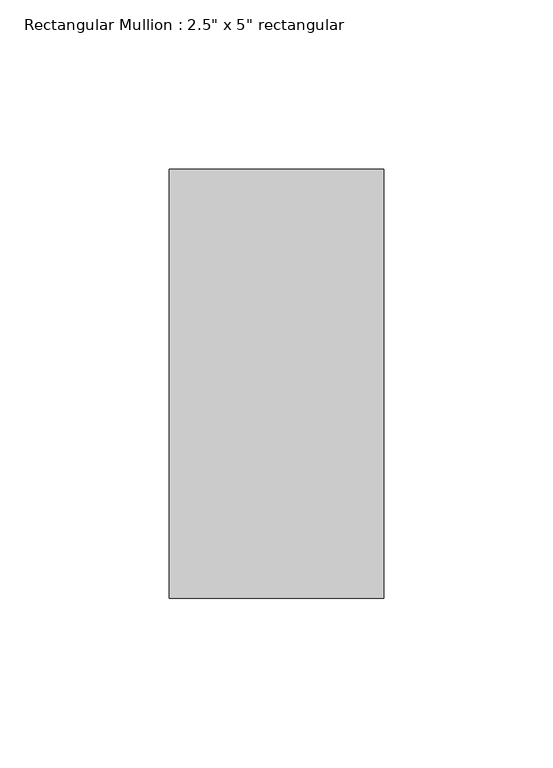
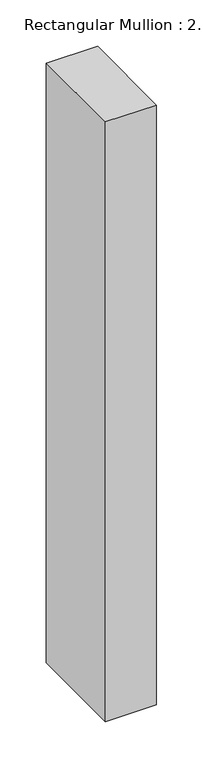
"""IFC4 building model written with IfcOpenShell, lengths in millimetres: member geometry."""

from ifc_helpers import new_model, si_unit, frame, origin, place, context, project, spatial, polyline, outline, extrude, source, transform, mapped, element, save


def member_24b317d4(model_context):
    return source(origin(), model_context, "Body", "SweptSolid", [
        extrude(outline(polyline([(31.75, 63.5), (31.75, -63.5), (-31.75, -63.5), (-31.75, 63.5), (31.75, 63.5)])), frame((0.0, 0.0, -788.0989237), z_axis=(0.0, 0.0, 1.0), x_axis=(1.0, 0.0, 0.0)), (0.0, 0.0, 1.0), 788.0989237),
    ])


if __name__ == "__main__":
    model = new_model("IFC4")
    model_context = context("Model", 3, world=origin())
    ifc_project = project(units=[si_unit("LENGTHUNIT", "METRE", prefix="MILLI")], contexts=[model_context])
    site = spatial("IfcSite", under=ifc_project)
    building = spatial("IfcBuilding", under=site)
    placement = place(None, origin())
    member_shape = member_24b317d4(model_context)
    element("IfcMember", 1, ObjectType="Rectangular Mullion : 2.5\" x 5\" rectangular", at=placement, inside=building, context=model_context, shape_type="MappedRepresentation", body=[
        mapped(member_shape, transform((0.0, 0.0, 0.0), x_axis=(1.0, 0.0, 0.0), y_axis=(0.0, 1.0, 0.0), z_axis=(0.0, 0.0, 1.0))),
    ])
    save(model, "model.ifc")

# Revit data of these elements
# Type "Rectangular Mullion : 2.5\" x 5\" rectangular"
#   built-in parameter 1007304 = 0.416667 (stored number, unit not read)
#   built-in parameter 1007301 = 0.104167 (stored number, unit not read)
#   built-in parameter 1007300 = 0.104167 (stored number, unit not read)
# Element 1 (IfcMember, "Rectangular Mullion : 2.5\" x 5\" rectangular")
#   Materials on its faces: "Aluminum"
# Materials
#   "Aluminum": class "Metal", colour RGB 247 247 247, transparency 0, Description = "Aluminum 6061", Cost = 0
